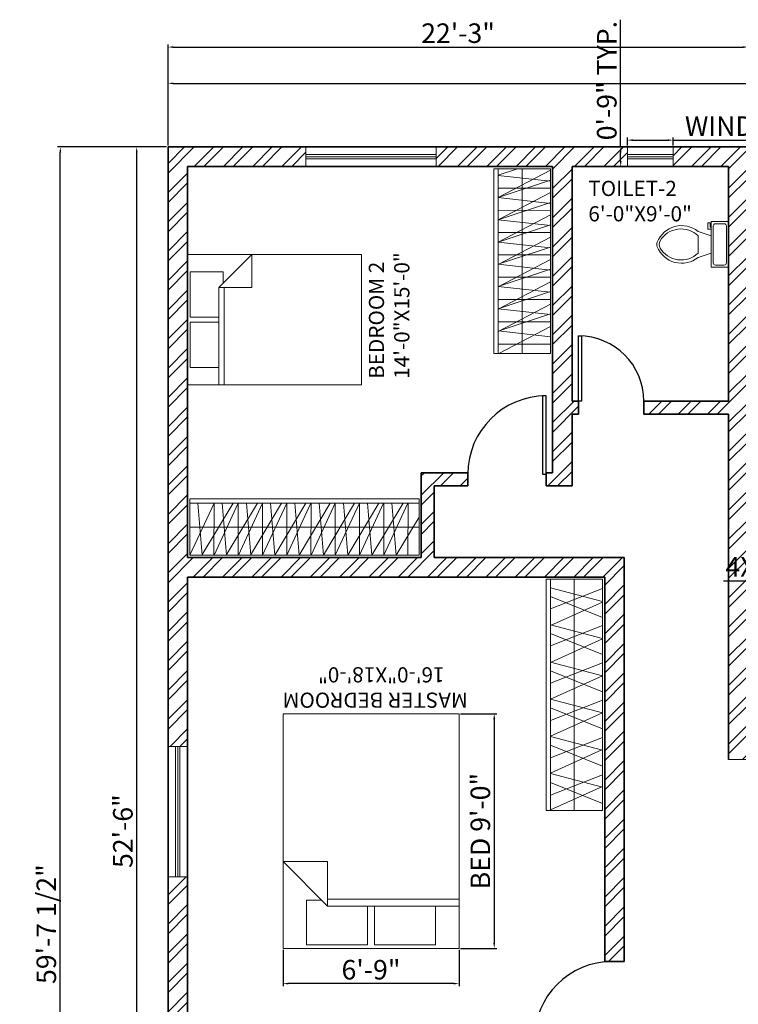
# Model space of a CAD drawing. Units: inches. Extents: x 416 to 1422, y 799 to 1634.
# Tile 2 of 5: x 416 to 746, y 1174 to 1628. Entities that reach past the tile are written whole.
import ezdxf

# ---------------------------------------------------------------- set-up
doc = ezdxf.new("R2010")
doc.units = ezdxf.units.IN
doc.linetypes.add('ACAD_ISO02W100', pattern=[15, 12, -3])
for name, color, linetype, lineweight in [('A-ANNO-DIMS', 2, 'Continuous', 18), ('A-AREA-IDEN', 7, 'Continuous', 18), ('A-DOOR', 4, 'Continuous', 25), ('A-FLOR-CASE', 8, 'Continuous', 18), ('A-FLOR-CASE-PATT', 252, 'Continuous', 13), ('A-FLOR-FIXT', 9, 'Continuous', 18), ('A-FURN', 8, 'Continuous', 18), ('A-GLAZ', 244, 'Continuous', 18), ('A-WALL', 7, 'Continuous', 35), ('A-WALL-HIDN', 7, 'ACAD_ISO02W100', 18), ('A-WALL-PATT', 252, 'Continuous', 13)]:
    doc.layers.add(name, color=color, linetype=linetype, lineweight=lineweight)
doc.styles.get("Standard").update_dxf_attribs({"font": 'arial.ttf'})
doc.dimstyles.new('ISO-25', dxfattribs={"dimtxt": 9, "dimasz": 2.5, "dimexe": 1.25, "dimexo": 0.625, "dimtad": 1, "dimlunit": 3, "dimtxsty": 'Standard', "dimcen": 2.5, "dimadec": 0, "dimazin": 0, "dimtfac": 1, "dimtmove": 0, "dimatfit": 3, "dimfxl": 1, "dimarcsym": 0})

# ---------------------------------------------------------------- blocks, each defined once
blk = doc.blocks.new('*U2')
for p, q in [((0, 0), (0, -6)), ((40, 0), (40, -6))]:
    blk.add_line(p, q)
blk.add_lwpolyline([(0, 0), (0, 40), (1.75, 40), (1.75, 0)], close=True)
blk.add_arc((0, 0), 40, 0, 90)
blk = doc.blocks.new('*U8')
for p, q in [((0, 0), (0, -6)), ((-40, 0), (-40, -6))]:
    blk.add_line(p, q)
blk.add_lwpolyline([(0, 0), (0, 40), (-1.75, 40), (-1.75, 0)], close=True)
blk.add_arc((0, 0), 40, 90, 180)
blk = doc.blocks.new('*U5')
for p, q in [((0, 0), (0, -6)), ((40, 0), (40, -6))]:
    blk.add_line(p, q)
blk.add_lwpolyline([(0, 0), (0, 40), (1.75, 40), (1.75, 0)], close=True)
blk.add_arc((0, 0), 40, 0, 90)
blk = doc.blocks.new('*U7')
for p, q in [((9.5, -6), (9.5, -2)), ((-10, -8.5), (-8, -8.5)), ((-10, -9.5), (-10, -8.5)), ((-8, -8.5), (-8, -8)), ((-7, -8), (-7, -9.5)), ((-4, -8), (-6, -14)), ((4, -8), (6, -14)), ((-7, -9.5), (-10, -9.5)), ((4, -14), (-4, -14))]:
    blk.add_line(p, q)
blk.add_lwpolyline([(10.5, -8), (10.5, 0), (-10.5, 0), (-10.5, -8)], close=True)
for points in [[(-9.5, -2), (-9.5, -6)], [(8.5, -1), (-8.5, -1)], [(-8.5, -7), (8.5, -7)]]:
    blk.add_lwpolyline(points)
for centre, radius, start, end in [((-8.62, -1.88), 0.884, 81.8699, 188.1301), ((8.62, -1.88), 0.884, 351.8699, 98.1301), ((-8.62, -6.12), 0.884, 171.8699, 278.1301), ((8.62, -6.12), 0.884, 261.8699, 8.1301), ((3.52, -21.58), 12.17, 141.4691, 247.9714), ((4.2, -21.82), 11.33, 136.3677, 238.9468), ((-3.52, -21.58), 12.17, 292.0284, 38.5307), ((-4.2, -21.82), 11.33, 301.053, 43.6321), ((0, -27.88), 4, 245.7318, 294.2682), ((0, -29), 4, 254.8605, 285.1395)]:
    blk.add_arc(centre, radius, start, end)
blk = doc.blocks.new('Bed - Queen')
for p, q in [((0, -80.00003), (0, 0)), ((0, 0), (59.99999, 0)), ((59.99999, 0), (59.99999, -80.00003)), ((7.99999, -1.2), (28.79998, -1.2)), ((7.99999, -14.4), (7.99999, -1.2)), ((28.79998, -1.2), (28.79998, -14.4)), ((31.19999, -1.2), (51.99999, -1.2)), ((31.19999, -14.4), (31.19999, -1.2)), ((51.99999, -1.2), (51.99999, -16.4)), ((0, -14.4), (44.8, -14.4)), ((59.99999, -29.6), (44.8, -14.4)), ((44.8, -14.4), (44.8, -29.6)), ((51.99999, -16.4), (46.79936, -16.4)), ((44.8, -16.8), (0, -16.8)), ((44.8, -29.6), (59.99999, -29.6)), ((59.99999, -80.00003), (0, -80.00003))]:
    blk.add_line(p, q)
blk = doc.blocks.new('*D16')
at = {"layer": 'A-ANNO-DIMS', "color": 0, "lineweight": -2, "transparency": 16777216}
for p, q in [((483.19, 1569.01), (468.17, 1569.01)), ((469.42, 941.51), (469.42, 1566.51)), ((483.19, 939.01), (468.17, 939.01))]:
    blk.add_line(p, q, dxfattribs=at)
at = {"layer": 'A-ANNO-DIMS', "color": 0, "transparency": 16777216}
for points in [[(469, 1566.51), (469.84, 1566.51), (469.42, 1569.01)], [(469, 941.51), (469.84, 941.51), (469.42, 939.01)]]:
    blk.add_solid(points, dxfattribs=at)
at = {"layer": 'Defpoints', "color": 0, "transparency": 16777216}
for p in [(469.42, 1569.01), (483.82, 1569.01), (483.82, 939.01)]:
    blk.add_point(p, dxfattribs=at)
at = {"layer": 'A-ANNO-DIMS', "color": 0, "transparency": 16777216, "insert": (464.2, 1254.01), "char_height": 9, "attachment_point": 5, "rotation": 90}
blk.add_mtext('52\'-6"', dxfattribs=at)
blk = doc.blocks.new('*D17')
at = {"layer": 'A-ANNO-DIMS', "color": 0, "lineweight": -2, "transparency": 16777216}
for p, q in [((483.82, 1569.64), (483.82, 1599.55)), ((486.32, 1598.3), (1321.32, 1598.3)), ((1323.82, 1569.64), (1323.82, 1599.55))]:
    blk.add_line(p, q, dxfattribs=at)
at = {"layer": 'A-ANNO-DIMS', "color": 0, "transparency": 16777216}
for points in [[(486.32, 1598.72), (486.32, 1597.88), (483.82, 1598.3)], [(1321.32, 1598.72), (1321.32, 1597.88), (1323.82, 1598.3)]]:
    blk.add_solid(points, dxfattribs=at)
at = {"layer": 'Defpoints', "color": 0, "transparency": 16777216}
for p in [(1323.82, 1598.3), (483.82, 1569.01), (1323.82, 1569.01)]:
    blk.add_point(p, dxfattribs=at)
at = {"layer": 'A-ANNO-DIMS', "color": 0, "transparency": 16777216, "insert": (903.82, 1603.52), "char_height": 9, "attachment_point": 5}
blk.add_mtext("70'", dxfattribs=at)
blk = doc.blocks.new('WIN-21IN')
for p, q in [((21, 5.5), (0, 5.5)), ((21, 4.5), (0, 4.5)), ((21, 3.5), (0, 3.5))]:
    blk.add_line(p, q)
blk.add_lwpolyline([(21, 9), (21, 0), (0, 0), (0, 9)], close=True)
blk = doc.blocks.new('WIN-60IN')
for p, q in [((3.5, 60), (3.5, 0)), ((4.5, 60), (4.5, 0)), ((5.5, 60), (5.5, 0))]:
    blk.add_line(p, q)
blk.add_lwpolyline([(0, 60), (9, 60), (9, 0), (0, 0)], close=True)
blk = doc.blocks.new('*D25')
at = {"layer": 'A-ANNO-DIMS', "color": 0, "lineweight": -2, "transparency": 16777216}
for p, q in [((695.32, 1569.64), (695.32, 1573.41)), ((716.32, 1569.64), (716.32, 1573.41)), ((697.82, 1572.16), (713.82, 1572.16)), ((716.32, 1572.16), (833.96, 1572.16))]:
    blk.add_line(p, q, dxfattribs=at)
at = {"layer": 'A-ANNO-DIMS', "color": 0, "transparency": 16777216}
for points in [[(697.82, 1572.58), (697.82, 1571.75), (695.32, 1572.16)], [(713.82, 1572.58), (713.82, 1571.75), (716.32, 1572.16)]]:
    blk.add_solid(points, dxfattribs=at)
at = {"layer": 'Defpoints', "color": 0, "transparency": 16777216}
for p in [(695.32, 1569.01), (716.32, 1572.16), (716.32, 1569.01)]:
    blk.add_point(p, dxfattribs=at)
at = {"layer": 'A-ANNO-DIMS', "color": 0, "transparency": 16777216, "insert": (776.39, 1577.44), "char_height": 9, "attachment_point": 5}
blk.add_mtext('WINDOW 1\'-9" TYP.', dxfattribs=at)
blk = doc.blocks.new('*D26')
at = {"layer": 'A-ANNO-DIMS', "color": 0, "lineweight": -2, "transparency": 16777216}
for p, q in [((692.17, 1569.01), (692.17, 1627.62)), ((694.69, 1569.01), (690.92, 1569.01)), ((692.17, 1562.51), (692.17, 1566.51)), ((694.69, 1560.01), (690.92, 1560.01))]:
    blk.add_line(p, q, dxfattribs=at)
at = {"layer": 'A-ANNO-DIMS', "color": 0, "transparency": 16777216}
for points in [[(691.75, 1566.51), (692.59, 1566.51), (692.17, 1569.01)], [(691.75, 1562.51), (692.59, 1562.51), (692.17, 1560.01)]]:
    blk.add_solid(points, dxfattribs=at)
at = {"layer": 'Defpoints', "color": 0, "transparency": 16777216}
for p in [(692.17, 1569.01), (695.32, 1569.01), (695.32, 1560.01)]:
    blk.add_point(p, dxfattribs=at)
at = {"layer": 'A-ANNO-DIMS', "color": 0, "transparency": 16777216, "insert": (686.95, 1599.57), "char_height": 9, "attachment_point": 5, "rotation": 90}
blk.add_mtext('0\'-9" TYP.', dxfattribs=at)
blk = doc.blocks.new('*D31')
at = {"layer": 'A-ANNO-DIMS', "color": 0, "lineweight": -2, "transparency": 16777216}
for p, q in [((618.39, 1308.05), (635.22, 1308.05)), ((633.97, 1305.55), (633.97, 1202.52)), ((618.39, 1200.02), (635.22, 1200.02))]:
    blk.add_line(p, q, dxfattribs=at)
at = {"layer": 'A-ANNO-DIMS', "color": 0, "transparency": 16777216}
for points in [[(633.56, 1305.55), (634.39, 1305.55), (633.97, 1308.05)], [(633.56, 1202.52), (634.39, 1202.52), (633.97, 1200.02)]]:
    blk.add_solid(points, dxfattribs=at)
at = {"layer": 'Defpoints', "color": 0, "transparency": 16777216}
for p in [(617.77, 1308.05), (617.77, 1200.02), (633.97, 1200.02)]:
    blk.add_point(p, dxfattribs=at)
at = {"layer": 'A-ANNO-DIMS', "color": 0, "transparency": 16777216, "insert": (628.75, 1254.03), "char_height": 9, "attachment_point": 5, "rotation": 90}
blk.add_mtext('BED 9\'-0"', dxfattribs=at)
blk = doc.blocks.new('*D32')
at = {"layer": 'A-ANNO-DIMS', "color": 0, "lineweight": -2, "transparency": 16777216}
for p, q in [((536.75, 1199.39), (536.75, 1182.56)), ((617.77, 1199.39), (617.77, 1182.56)), ((615.27, 1183.81), (539.25, 1183.81))]:
    blk.add_line(p, q, dxfattribs=at)
at = {"layer": 'A-ANNO-DIMS', "color": 0, "transparency": 16777216}
for points in [[(539.25, 1184.23), (539.25, 1183.39), (536.75, 1183.81)], [(615.27, 1184.23), (615.27, 1183.39), (617.77, 1183.81)]]:
    blk.add_solid(points, dxfattribs=at)
at = {"layer": 'Defpoints', "color": 0, "transparency": 16777216}
for p in [(536.75, 1200.02), (617.77, 1200.02), (536.75, 1183.81)]:
    blk.add_point(p, dxfattribs=at)
at = {"layer": 'A-ANNO-DIMS', "color": 0, "transparency": 16777216, "insert": (577.26, 1189.03), "char_height": 9, "attachment_point": 5}
blk.add_mtext('6\'-9"', dxfattribs=at)
blk = doc.blocks.new('*D43')
at = {"layer": 'A-ANNO-DIMS', "color": 0, "lineweight": -2, "transparency": 16777216}
for p, q in [((483.19, 1569.01), (433, 1569.01)), ((434.25, 855.88), (434.25, 1566.51)), ((909.15, 853.38), (433, 853.38))]:
    blk.add_line(p, q, dxfattribs=at)
at = {"layer": 'A-ANNO-DIMS', "color": 0, "transparency": 16777216}
for points in [[(433.83, 1566.51), (434.67, 1566.51), (434.25, 1569.01)], [(433.83, 855.88), (434.67, 855.88), (434.25, 853.38)]]:
    blk.add_solid(points, dxfattribs=at)
at = {"layer": 'Defpoints', "color": 0, "transparency": 16777216}
for p in [(434.25, 1569.01), (483.82, 1569.01), (909.77, 853.38)]:
    blk.add_point(p, dxfattribs=at)
at = {"layer": 'A-ANNO-DIMS', "color": 0, "transparency": 16777216, "insert": (428.97, 1211.2), "char_height": 9, "attachment_point": 5, "rotation": 90}
blk.add_mtext('59\'-7 1/2"', dxfattribs=at)
blk = doc.blocks.new('*D51')
at = {"layer": 'A-ANNO-DIMS', "color": 0, "lineweight": -2, "transparency": 16777216}
for p, q in [((483.82, 1569.64), (483.82, 1616.26)), ((486.32, 1615.01), (748.32, 1615.01)), ((750.82, 1569.64), (750.82, 1616.26))]:
    blk.add_line(p, q, dxfattribs=at)
at = {"layer": 'A-ANNO-DIMS', "color": 0, "transparency": 16777216}
for points in [[(486.32, 1615.43), (486.32, 1614.6), (483.82, 1615.01)], [(748.32, 1615.43), (748.32, 1614.6), (750.82, 1615.01)]]:
    blk.add_solid(points, dxfattribs=at)
at = {"layer": 'Defpoints', "color": 0, "transparency": 16777216}
for p in [(750.82, 1615.01), (483.82, 1569.01), (750.82, 1569.01)]:
    blk.add_point(p, dxfattribs=at)
at = {"layer": 'A-ANNO-DIMS', "color": 0, "transparency": 16777216, "insert": (617.32, 1620.24), "char_height": 9, "attachment_point": 5}
blk.add_mtext('22\'-3"', dxfattribs=at)
blk = doc.blocks.new('*D59')
at = {"layer": 'A-ANNO-DIMS', "color": 0, "lineweight": -2, "transparency": 16777216}
for p, q in [((739.52, 1369.23), (842.8, 1369.23)), ((959.55, 1369.23), (845.3, 1369.23))]:
    blk.add_line(p, q, dxfattribs=at)
at = {"layer": 'A-ANNO-DIMS', "color": 0, "transparency": 16777216}
blk.add_solid([(842.8, 1369.65), (842.8, 1368.81), (845.3, 1369.23)], dxfattribs=at)
at = {"layer": 'Defpoints', "color": 0, "transparency": 16777216}
for p in [(845.3, 1369.23), (959.55, 1369.23)]:
    blk.add_point(p, dxfattribs=at)
at = {"layer": 'A-ANNO-DIMS', "color": 0, "transparency": 16777216, "insert": (776.75, 1374.51), "char_height": 9, "attachment_point": 5, "rotation": 359.9998}
blk.add_mtext('4X R9\'-6 1/2"', dxfattribs=at)

msp = doc.modelspace()

# ---------------------------------------------------------------- hatches: boundary and pattern name
at = {"layer": 'A-FLOR-CASE-PATT'}
h = msp.add_hatch(dxfattribs=at)
h.set_pattern_fill('ANSI31', color=256, scale=2.86898, angle=-17.3791, style=0)
h.paths.add_polyline_path([(635.82, 1549.082), (635.82, 1473.964), (642.149, 1473.964), (659.82, 1483.132), (659.82, 1559.013), (654.961, 1559.013)])
h = msp.add_hatch(dxfattribs=at)
h.set_pattern_fill('ANSI31', color=256, scale=3.202738, angle=128.6367, style=0)
h.paths.add_polyline_path([(635.82, 1480.942), (659.82, 1478.265), (659.82, 1556.667), (638.787, 1559.013), (635.82, 1559.013)])
h = msp.add_hatch(dxfattribs=at)
h.set_pattern_fill('ANSI31', color=256, scale=3.0698, angle=-26.652, style=0)
h.paths.add_polyline_path([(635.82, 1480.942), (659.82, 1488.849), (659.82, 1559.013), (635.82, 1559.013)])
h = msp.add_hatch(dxfattribs=at)
h.set_pattern_fill('ANSI31', color=256, scale=3.23213, angle=-44.9528, style=0)
h.paths.add_polyline_path([(635.82, 1553.382), (635.82, 1474.981), (659.82, 1474.981), (659.82, 1553.382)])
h = msp.add_hatch(dxfattribs=at)
h.set_pattern_fill('ANSI31', color=256, scale=3.18747, angle=20.175, style=0)
h.paths.add_polyline_path([(493.82, 1388.693), (493.82, 1381.013), (586.68, 1381.013), (597.841, 1405.013), (501.409, 1405.013)])
h = msp.add_hatch(dxfattribs=at)
h.set_pattern_fill('ANSI31', color=256, scale=3.50285, angle=49.728, style=0)
h.paths.add_polyline_path([(495.998, 1381.013), (592.429, 1381.013), (590.406, 1405.013), (493.974, 1405.013)])
h = msp.add_hatch(dxfattribs=at)
h.set_pattern_fill('ANSI31', color=256, scale=3.02446, angle=14.1865, style=0)
h.paths.add_polyline_path([(495.998, 1381.013), (592.429, 1381.013), (599.403, 1392.786), (599.403, 1405.013), (510.215, 1405.013)])
h = msp.add_hatch(dxfattribs=at)
h.set_pattern_fill('ANSI31', color=256, scale=3.51528, angle=44.8876, style=0)
h.paths.add_polyline_path([(501.409, 1381.013), (597.841, 1381.013), (597.841, 1405.013), (501.409, 1405.013)])
h = msp.add_hatch(dxfattribs=at)
h.set_pattern_fill('ANSI31', color=256, scale=5.0388, angle=-23.689, style=0)
h.paths.add_polyline_path([(659.82, 1361.7), (659.82, 1265.395), (683.82, 1274.757), (683.82, 1370.013), (681.128, 1370.013)])
h = msp.add_hatch(dxfattribs=at)
h.set_pattern_fill('ANSI31', color=256, scale=5.21012, angle=120.292, style=0)
h.paths.add_polyline_path([(659.82, 1275.105), (683.82, 1268.805), (683.82, 1365.11), (665.145, 1370.013), (659.82, 1370.013)])
h = msp.add_hatch(dxfattribs=at)
h.set_pattern_fill('ANSI31', color=256, scale=5.00607, angle=113.072, style=0)
h.paths.add_polyline_path([(659.82, 1367.384), (659.82, 1271.078), (678.661, 1263.493), (683.82, 1263.493), (683.82, 1357.722)])
h = msp.add_hatch(dxfattribs=at)
h.set_pattern_fill('ANSI31', color=256, scale=4.8773, angle=-20.821, style=0)
h.paths.add_polyline_path([(659.82, 1354.335), (659.82, 1263.493), (671.99, 1263.493), (683.82, 1268.805), (683.82, 1365.11)])
at = {"layer": 'A-WALL-PATT'}
h = msp.add_hatch(dxfattribs=at)
h.set_pattern_fill('ANSI32', color=256)
h.paths.add_polyline_path([(726.961, 969.013), (653.32, 969.013), (653.32, 975.013), (644.32, 975.013), (644.32, 939.013), (653.32, 939.013), (653.32, 960.013), (726.961, 960.013)])
h.paths.add_polyline_path([(929.602, 967.213), (929.602, 969.013), (917.602, 969.013), (917.602, 1089.013), (908.602, 1089.013), (908.602, 969.013), (834.961, 969.013), (834.961, 960.013), (929.602, 960.013)])
h.paths.add_polyline_path([(693.82, 1158.013), (684.82, 1158.013), (684.82, 1155.013), (651.82, 1155.013), (651.82, 1146.013), (684.82, 1146.013), (684.82, 1050.013), (594.82, 1050.013), (594.82, 1102.56), (588.82, 1102.56), (588.82, 1026.013), (492.82, 1026.013), (492.82, 1035.612), (483.82, 1035.612), (483.82, 1017.013), (594.82, 1017.013), (594.82, 1041.013), (644.32, 1041.013), (644.32, 1035.013), (653.32, 1035.013), (653.32, 1041.013), (693.82, 1041.013)])
h.paths.add_polyline_path([(603.82, 1155.013), (492.82, 1155.013), (492.82, 1233.013), (483.82, 1233.013), (483.82, 1056.612), (492.82, 1056.612), (492.82, 1146.013), (588.82, 1146.013), (588.82, 1132.56), (594.82, 1132.56), (594.82, 1146.013), (603.82, 1146.013)])
h.paths.add_polyline_path([(693.82, 1380.013), (606.403, 1380.013), (606.403, 1413.013), (621.82, 1413.013), (621.82, 1419.013), (600.403, 1419.013), (600.403, 1380.013), (492.82, 1380.013), (492.82, 1419.013), (492.82, 1560.013), (547.303, 1560.013), (547.303, 1569.013), (483.82, 1569.013), (483.82, 1293.013), (492.82, 1293.013), (492.82, 1371.013), (684.82, 1371.013), (684.82, 1194.013), (693.82, 1194.013)])
h = msp.add_hatch(dxfattribs=at)
h.set_pattern_fill('ANSI32', color=256)
h.paths.add_polyline_path([(695.32, 1569.013), (607.303, 1569.013), (607.303, 1560.013), (660.82, 1560.013), (660.82, 1419.013), (657.82, 1419.013), (657.82, 1413.013), (669.82, 1413.013), (669.82, 1446.013), (672.82, 1446.013), (672.82, 1452.013), (669.82, 1452.013), (669.82, 1560.013), (695.32, 1560.013)])
h.paths.add_polyline_path([(1323.82, 1311.283), (1314.82, 1311.283), (1314.82, 1287.013), (1242.82, 1287.013), (1242.82, 1383.013), (1245.82, 1383.013), (1245.82, 1392.013), (1236.82, 1392.013), (1236.82, 1339.513), (1158.82, 1339.513), (1158.82, 1431.013), (1149.82, 1431.013), (1149.82, 1287.013), (1044.82, 1287.013), (1044.82, 1242.013), (1053.82, 1242.013), (1053.82, 1278.013), (1221.82, 1278.013), (1221.82, 1233.013), (1230.82, 1233.013), (1230.82, 1278.013), (1314.82, 1278.013), (1314.82, 1225.894), (1323.82, 1225.894)])
h.paths.add_polyline_path([(1158.82, 1287.013), (1158.82, 1333.513), (1236.82, 1333.513), (1236.82, 1287.013)], flags=16)
h.paths.add_polyline_path([(1323.82, 1569.013), (1283.747, 1569.013), (1283.747, 1560.013), (1314.82, 1560.013), (1314.82, 1392.013), (1275.82, 1392.013), (1275.82, 1383.013), (1314.82, 1383.013), (1314.82, 1332.283), (1323.82, 1332.283)])
h.paths.add_polyline_path([(750.82, 1569.013), (716.32, 1569.013), (716.32, 1560.013), (741.82, 1560.013), (741.82, 1452.013), (702.82, 1452.013), (702.82, 1447.513), (702.82, 1446.013), (741.82, 1446.013), (741.82, 1287.013), (750.82, 1287.013)])
h.paths.add_polyline_path([(1158.82, 1560.013), (1223.747, 1560.013), (1223.747, 1569.013), (1149.82, 1569.013), (1149.82, 1467.013), (1158.82, 1467.013)])
h.paths.add_polyline_path([(1323.82, 1098.013), (1230.82, 1098.013), (1230.82, 1149.013), (1323.82, 1149.013), (1323.82, 1204.894), (1314.82, 1204.894), (1314.82, 1158.013), (1230.82, 1158.013), (1230.82, 1203.013), (1221.82, 1203.013), (1221.82, 1098.013), (1053.82, 1098.013), (1053.82, 1194.013), (1044.82, 1194.013), (1044.82, 1089.013), (1104.82, 1089.013), (1104.82, 1086.013), (1113.82, 1086.013), (1113.82, 1089.013), (1194.82, 1089.013), (1314.82, 1089.013), (1314.82, 897.013), (1194.82, 897.013), (1194.82, 1041.013), (1113.82, 1041.013), (1113.82, 1044.013), (1104.82, 1044.013), (1104.82, 1032.013), (1113.82, 1032.013), (1113.82, 1035.013), (1185.82, 1035.013), (1185.82, 969.013), (1113.82, 969.013), (1113.82, 1008.013), (1104.82, 1008.013), (1104.82, 969.013), (1088.452, 969.013), (1088.452, 960.013), (1185.82, 960.013), (1185.82, 888.013), (1323.82, 888.013)])

# ---------------------------------------------------------------- linework, layer by layer
at = {"layer": 'A-FLOR-CASE'}
for p, q in [((633.82, 1559.013), (659.82, 1559.013)), ((633.82, 1559.013), (633.82, 1473.964)), ((635.82, 1559.013), (635.82, 1473.964)), ((646.82, 1559.013), (646.82, 1473.964)), ((659.82, 1559.013), (659.82, 1473.964)), ((659.82, 1473.964), (633.82, 1473.964)), ((493.82, 1407.013), (493.82, 1381.013)), ((493.82, 1407.013), (599.403, 1407.013)), ((599.403, 1381.013), (599.403, 1407.013)), ((493.82, 1405.013), (599.403, 1405.013)), ((493.82, 1394.013), (599.403, 1394.013)), ((493.82, 1381.013), (599.403, 1381.013)), ((657.82, 1370.013), (683.82, 1370.013)), ((657.82, 1370.013), (657.82, 1263.493)), ((659.82, 1370.013), (659.82, 1263.493)), ((670.82, 1370.013), (670.82, 1263.493)), ((683.82, 1370.013), (683.82, 1263.493)), ((683.82, 1263.493), (657.82, 1263.493))]:
    msp.add_line(p, q, dxfattribs=at)
at = {"layer": 'A-WALL'}
for p, q in [((483.82, 1569.013), (483.82, 939.013)), ((483.82, 1569.013), (1323.82, 1569.013)), ((492.82, 1560.013), (492.82, 1419.013)), ((492.82, 1560.013), (660.82, 1560.013)), ((660.82, 1560.013), (660.82, 1419.013)), ((669.82, 1560.013), (669.82, 1452.013)), ((669.82, 1560.013), (741.82, 1560.013)), ((741.82, 1560.013), (741.82, 1452.013)), ((669.82, 1452.013), (672.82, 1452.013)), ((672.82, 1446.013), (672.82, 1452.013)), ((702.82, 1446.013), (702.82, 1452.013)), ((702.82, 1452.013), (741.82, 1452.013)), ((669.82, 1446.013), (672.82, 1446.013)), ((669.82, 1446.013), (669.82, 1413.013)), ((702.82, 1446.013), (741.82, 1446.013)), ((741.82, 1446.013), (741.82, 1287.013)), ((492.82, 1419.013), (492.82, 1380.013)), ((600.403, 1419.013), (621.82, 1419.013)), ((600.403, 1380.013), (600.403, 1419.013)), ((621.82, 1419.013), (621.82, 1413.013)), ((657.82, 1419.013), (657.82, 1413.013)), ((657.82, 1419.013), (660.82, 1419.013)), ((606.403, 1380.013), (606.403, 1413.013)), ((606.403, 1413.013), (621.82, 1413.013)), ((657.82, 1413.013), (669.82, 1413.013)), ((492.82, 1380.013), (600.403, 1380.013)), ((606.403, 1380.013), (693.82, 1380.013)), ((693.82, 1380.013), (693.82, 1194.013)), ((492.82, 1371.013), (684.82, 1371.013)), ((492.82, 1371.013), (492.82, 1155.013)), ((684.82, 1371.013), (684.82, 1194.013)), ((684.82, 1194.013), (693.82, 1194.013))]:
    msp.add_line(p, q, dxfattribs=at)
at = {"layer": 'A-WALL-HIDN'}
msp.add_line((750.82, 1287.013), (741.82, 1287.013), dxfattribs=at)

# ---------------------------------------------------------------- block references
at = {"layer": 'A-DOOR'}
for name, p, xscale, yscale, zscale in [('*U5', (672.82, 1452.013), 0.75, 0.75, 0.75), ('*U8', (657.82, 1418.413), 0.8999999999999942, 0.8999999999999942, 0.8999999999999942)]:
    msp.add_blockref(name, p, dxfattribs=dict(at, xscale=xscale, yscale=yscale, zscale=zscale))
at = {"layer": 'A-DOOR', "xscale": 0.8999999999999942, "yscale": 0.8999999999999942, "zscale": 0.8999999999999942, "rotation": 89.99999999999994}
msp.add_blockref('*U2', (688.42, 1158.013), dxfattribs=at)
at = {"layer": 'A-FLOR-FIXT', "rotation": 270}
msp.add_blockref('*U7', (741.82, 1524.146), dxfattribs=at)
at = {"layer": 'A-FURN', "rotation": 90}
msp.add_blockref('Bed - Queen', (492.82, 1459.513), dxfattribs=at)
at = {"layer": 'A-FURN', "xscale": 1.350376073941423, "yscale": 1.350376073941423, "zscale": 1.350376073941423, "rotation": 180}
msp.add_blockref('Bed - Queen', (617.77, 1200.015), dxfattribs=at)
at = {"layer": 'A-GLAZ', "rotation": 270.0000000000007}
msp.add_blockref('WIN-60IN', (547.303, 1569.012), dxfattribs=at)
at = {"layer": 'A-GLAZ'}
for name, p in [('WIN-21IN', (695.32, 1560.013)), ('WIN-60IN', (483.82, 1233.013))]:
    msp.add_blockref(name, p, dxfattribs=at)

# ---------------------------------------------------------------- texts
at = {"layer": 'A-AREA-IDEN', "insert": (677.283, 1553.431), "char_height": 7, "attachment_point": 1}
msp.add_mtext_dynamic_manual_height_columns('TOILET-2 \\P6\'-0"X9\'-0"', width=44.45572, gutter_width=12.5, heights=[0], dxfattribs=at)
at = {"layer": 'A-AREA-IDEN', "char_height": 7, "attachment_point": 1}
for s, width, insert, rotation in [('BEDROOM 2\\P14\'-0"X15\'-0"', 62.77808, (576.263, 1462.27), 90), ('MASTER BEDROOM\\P     16\'-0"X18\'-0"', 94.81104, (621.813, 1310.803), 180)]:
    msp.add_mtext_dynamic_manual_height_columns(s, width=width, gutter_width=12.5, heights=[0], dxfattribs=dict(at, insert=insert, rotation=rotation))

# ---------------------------------------------------------------- dimensions: what is measured, and where the dimension line sits
at = {"layer": 'A-ANNO-DIMS'}
for base, p1, p2, angle, text, picture, middle in [((692.17, 1569.013), (695.32, 1560.013), (695.32, 1569.013), 90, '<> TYP.', '*D26', (686.95, 1599.567)), ((633.974, 1200.015), (617.77, 1308.045), (617.77, 1200.015), 270, 'BED <>', '*D31', (628.754, 1254.03))]:
    dim = msp.add_linear_dim(base=base, p1=p1, p2=p2, angle=angle, text=text, dimstyle='ISO-25', override={"dimdec": 1, "dimlfac": 1, "dimrnd": 0, "dimzin": 1, "dimdsep": 46, "dimlunit": 4, "dimfrac": 2}, dxfattribs=at)
    dim.commit()
    dim.dimension.update_dxf_attribs({"geometry": picture, "text_midpoint": middle})
for base, p2, override, picture, middle in [((750.82, 1615.013), (750.82, 1569.013), {"dimdec": 1, "dimlfac": 1, "dimrnd": 0, "dimzin": 1, "dimdsep": 46, "dimlunit": 4, "dimfrac": 2}, '*D51', (617.32, 1620.236)), ((1323.82, 1598.301), (1323.82, 1569.013), {"dimclrd": 0, "dimclre": 0, "dimclrt": 0}, '*D17', (903.82, 1603.522))]:
    dim = msp.add_linear_dim(base=base, p1=(483.82, 1569.013), p2=p2, dimstyle='ISO-25', override=override, dxfattribs=at)
    dim.commit()
    dim.dimension.update_dxf_attribs({"geometry": picture, "text_midpoint": middle})
dim = msp.add_linear_dim(base=(716.32, 1572.163), p1=(695.32, 1569.013), p2=(716.32, 1569.013), text='WINDOW <> TYP.', dimstyle='ISO-25', override={"dimdec": 1, "dimlfac": 1, "dimrnd": 0, "dimzin": 1, "dimdsep": 46, "dimlunit": 4, "dimfrac": 2}, dxfattribs=at)
dim.commit()
dim.dimension.update_dxf_attribs({"geometry": '*D25', "text_midpoint": (776.389, 1577.444)})
for base, p1, p2, angle, override, picture, middle in [((434.249, 1569.013), (909.773, 853.38), (483.82, 1569.013), 90, {"dimdec": 1, "dimlfac": 1, "dimrnd": 0, "dimzin": 1, "dimdsep": 46, "dimlunit": 4, "dimfrac": 2}, '*D43', (428.97, 1211.196)), ((469.419, 1569.013), (483.82, 939.013), (483.82, 1569.013), 90, {"dimclrd": 0, "dimclre": 0, "dimclrt": 0}, '*D16', (464.199, 1254.013)), ((536.747, 1183.811), (617.77, 1200.015), (536.747, 1200.015), 180, {"dimdec": 1, "dimlfac": 1, "dimrnd": 0, "dimzin": 1, "dimdsep": 46, "dimlunit": 4, "dimfrac": 2}, '*D32', (577.258, 1189.031))]:
    dim = msp.add_linear_dim(base=base, p1=p1, p2=p2, angle=angle, dimstyle='ISO-25', override=override, dxfattribs=at)
    dim.commit()
    dim.dimension.update_dxf_attribs({"geometry": picture, "text_midpoint": middle})
dim = msp.add_radius_dim(center=(959.546124, 1369.230665), mpoint=(845.296124, 1369.231), text='4X <>', dimstyle='ISO-25', override={"dimdec": 1, "dimlfac": 1, "dimrnd": 0, "dimzin": 1, "dimdsep": 46, "dimlunit": 4, "dimfrac": 2}, dxfattribs=at)
dim.commit()
dim.dimension.update_dxf_attribs({"geometry": '*D59', "text_midpoint": (776.746124, 1369.231201), "dimtype": 164})

doc.saveas('drawing.dxf')
